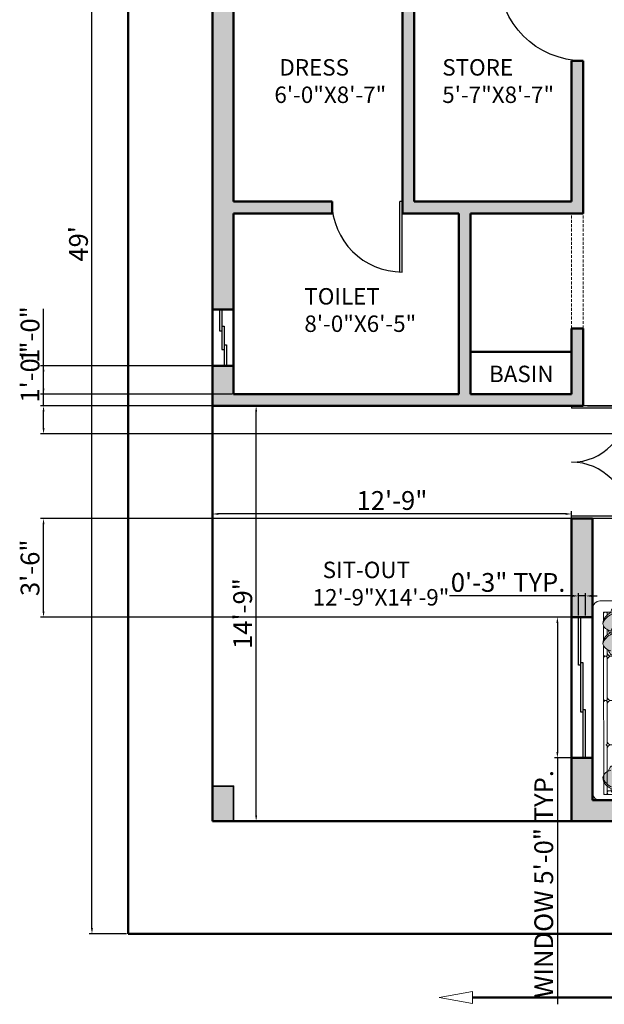
# Model space of a CAD drawing. Units: inches. Extents: x 1913 to 5309, y 1003 to 1733.
# Tile 9 of 23: x 2601 to 2850, y 1069 to 1488. Entities that reach past the tile are written whole.
import ezdxf

# ---------------------------------------------------------------- set-up
doc = ezdxf.new("R2010")
doc.units = ezdxf.units.IN
doc.linetypes.add('HIDDEN2', pattern=[0.1875, 0.125, -0.0625])
for name, color, linetype, lineweight in [('A-ANNO-DIMS', 2, 'Continuous', 18), ('A-ANNO-SYMB', 1, 'Continuous', 18), ('A-AREA-IDEN', 3, 'Continuous', 18), ('A-COLS', 5, 'Continuous', 35), ('A-COLS-PATT', 5, 'Continuous', 13), ('A-DOOR', 4, 'Continuous', 25), ('A-FLOR-PATT', 252, 'Continuous', 13), ('A-FURN', 8, 'Continuous', 18), ('A-GLAZ', 5, 'Continuous', 25), ('A-WALL', 7, 'Continuous', 50), ('A-WALL-OVHD', 8, 'HIDDEN2', 18)]:
    doc.layers.add(name, color=color, linetype=linetype, lineweight=lineweight)
doc.styles.get("Standard").update_dxf_attribs({"font": 'arial.ttf'})
doc.dimstyles.new('ISO-25', dxfattribs={"dimtxt": 8, "dimasz": 2.5, "dimexe": 1.25, "dimexo": 0.625, "dimtad": 1, "dimdec": 1, "dimlunit": 3, "dimtxsty": 'Standard', "dimcen": 2.5, "dimclrd": 256, "dimclrt": 1, "dimadec": 0, "dimazin": 0, "dimtfac": 1, "dimtdec": 1, "dimtmove": 0, "dimatfit": 3, "dimfxl": 1, "dimarcsym": 0})

# ---------------------------------------------------------------- blocks, each defined once
blk = doc.blocks.new('SOFA 1')
at = {"transparency": 33554687}
h = blk.add_hatch(color=256, dxfattribs=at)
h.dxf.hatch_style = 1
h.paths.add_polyline_path([(3723.52, 1308.63, 0.147724), (3717.76, 1305.24, 0.310469), (3722.42, 1300.4), (3722.42, 1300.25, 0.156703), (3723.62, 1297.8, 0.425821), (3734.69, 1309.08, 0.121928), (3732.05, 1310.63, 0.233216), (3728.6, 1313.59, 0.213835)])
h = blk.add_hatch(color=256, dxfattribs=at)
h.dxf.hatch_style = 1
h.paths.add_polyline_path([(3769.65, 1307.6, 0.084911), (3767.15, 1309.12, 0.046133), (3766.46, 1311.13), (3759.18, 1311.13, 0.039409), (3758.92, 1310.24, 0.165523), (3756.31, 1309.02, 0.42585), (3767.59, 1297.95, 0.121928), (3769.15, 1300.58, 0.027403), (3769.65, 1300.83)])
h.paths.add_polyline_path([(3765.34, 1313.08), (3760.4, 1313.08, 0.097704), (3759.18, 1311.13), (3766.46, 1311.13, 0.04873)])
h.paths.add_polyline_path([(3763.76, 1314.88, 0.16488), (3760.4, 1313.08), (3765.34, 1313.08, 0.051917)])
h.paths.add_polyline_path([(3771.6, 1305.17, 0.090388), (3769.65, 1307.6), (3769.65, 1300.83, 0.136035), (3771.6, 1302.77)])
h = blk.add_hatch(color=256, dxfattribs=at)
h.dxf.hatch_style = 1
h.paths.add_polyline_path([(3769.16, 1235.96, 0.122267), (3767.6, 1238.61, 0.425972), (3756.32, 1227.54, 0.165563), (3758.93, 1226.32, 0.309481), (3763.76, 1221.69, 0.002677), (3763.83, 1221.72, 0.146094), (3767.16, 1227.43, 0.212433), (3772.1, 1232.48, 0.235342)])
h = blk.add_hatch(color=256, dxfattribs=at)
h.dxf.hatch_style = 1
h.paths.add_polyline_path([(3769.16, 1225.36, 0.122267), (3767.6, 1228.01, 0.425972), (3756.32, 1216.94, 0.165563), (3758.93, 1215.72, 0.309481), (3763.76, 1211.09, 0.002677), (3763.83, 1211.12, 0.146094), (3767.16, 1216.83, 0.212433), (3772.1, 1221.88, 0.235342)])
for p, q in [((3720.45, 1316.13), (3773.58, 1316.13)), ((3777.51, 1312.19), (3777.51, 1213.72))]:
    blk.add_line(p, q, dxfattribs=at)
for points in [[(3717.76, 1305.24, -0.147724), (3723.52, 1308.63, -0.213355), (3728.59, 1313.59, 0.213355), (3723.52, 1308.63, 0.147724), (3717.76, 1305.24, -0.249545), (3722.86, 1309.34, 0.249545), (3717.75, 1305.25, 0.356779), (3723.4, 1300.28, -0.356779), (3717.76, 1305.24)], [(3728.58, 1313.6, -0.306333), (3732.42, 1309.31, 0.306333), (3728.58, 1313.6, 0.306674), (3722.72, 1308.89, -0.306674), (3728.58, 1313.6)], [(3763.76, 1314.88, -0.147724), (3767.15, 1309.12, -0.213355), (3772.1, 1304.05, 0.213355), (3767.15, 1309.12, 0.147724), (3763.76, 1314.88, -0.249545), (3767.86, 1309.77, 0.249545), (3763.77, 1314.89, 0.356779), (3758.8, 1309.23, -0.356779), (3763.76, 1314.88)], [(3734.69, 1309.08, -0.425972), (3723.62, 1297.8, -0.165552), (3722.4, 1300.4, 0.165552), (3723.62, 1297.79, 0.425972), (3734.69, 1309.07, 0.121514), (3732.07, 1310.63, -0.121514), (3734.69, 1309.08)], [(3767.6, 1297.95, -0.425972), (3756.31, 1309.01, -0.165552), (3758.92, 1310.24, 0.165552), (3756.31, 1309.02, 0.425972), (3767.59, 1297.95, 0.121514), (3769.14, 1300.57, -0.121514), (3767.6, 1297.95)], [(3772.11, 1304.06, -0.306333), (3767.83, 1300.22, 0.306333), (3772.11, 1304.06, 0.306674), (3767.4, 1309.91, -0.306674), (3772.11, 1304.06)], [(3770.44, 1286.63, -0.414214), (3769.66, 1287.4, 0.414214), (3770.44, 1286.63, 0.414214), (3769.66, 1285.83, -0.414214), (3770.44, 1286.63)], [(3748.01, 1262.99, -0.414214), (3746.05, 1264.95, 0.414214), (3748.01, 1262.97, 0.414213), (3746.05, 1261.01, -0.414213), (3748.01, 1262.99)], [(3770.44, 1262.99, -0.414214), (3769.66, 1263.77, 0.414214), (3770.44, 1262.99, 0.414214), (3769.66, 1262.19, -0.414214), (3770.44, 1262.99)], [(3770.83, 1262.97, -0.414214), (3771.61, 1262.19, 0.414214), (3770.83, 1262.99, 0.414214), (3771.61, 1263.77, -0.414214), (3770.83, 1262.97)], [(3748.01, 1239.35, -0.414214), (3746.05, 1241.31, 0.414214), (3748.01, 1239.33, 0.414213), (3746.05, 1237.37, -0.414213), (3748.01, 1239.35)], [(3767.7, 1239.33, -0.414214), (3769.66, 1237.37, 0.414214), (3767.7, 1239.35, 0.414214), (3769.66, 1241.31, -0.414214), (3767.7, 1239.33)], [(3770.44, 1239.35, -0.414214), (3769.66, 1240.13, 0.414214), (3770.44, 1239.33, 0.414214), (3769.66, 1238.55, -0.414214), (3770.44, 1239.35)], [(3770.83, 1239.33, -0.414214), (3771.61, 1238.55, 0.414214), (3770.83, 1239.35, 0.414214), (3771.61, 1240.13, -0.414214), (3770.83, 1239.33)], [(3756.32, 1227.54, -0.425972), (3767.6, 1238.61, -0.121514), (3769.16, 1235.98, 0.121514), (3767.6, 1238.61, 0.425972), (3756.32, 1227.54, 0.165552), (3758.93, 1226.32, -0.165552), (3756.32, 1227.54)], [(3772.1, 1232.5, -0.306674), (3767.41, 1226.64, 0.306674), (3772.1, 1232.5, 0.306333), (3767.84, 1236.34, -0.306333), (3772.1, 1232.5)], [(3763.78, 1221.67, 0.249545), (3767.87, 1226.78, -0.249545), (3763.76, 1221.69, -0.356779), (3758.81, 1227.32, 0.356779), (3763.77, 1221.68, 0.147724), (3767.16, 1227.43, 0.213355), (3772.11, 1232.51, -0.213355), (3767.16, 1227.43, -0.147724), (3763.78, 1221.67)], [(3756.32, 1216.94, -0.200233), (3759.49, 1224.76, 0.200233), (3756.32, 1216.94, 0.165552), (3758.93, 1215.72, -0.165552), (3756.32, 1216.94)], [(3772.1, 1221.9, -0.306674), (3767.41, 1216.04, 0.306674), (3772.1, 1221.9, -0.213355), (3767.16, 1216.83, -0.147724), (3763.77, 1211.08, 0.147724), (3767.15, 1216.83, 0.213355), (3772.1, 1221.9)], [(3763.76, 1211.09, -0.356779), (3758.81, 1216.72, 0.356779), (3763.76, 1211.09, 0.249545), (3767.87, 1216.18, -0.249545), (3763.76, 1211.09)]]:
    blk.add_lwpolyline(points, format="xyb", dxfattribs=at)
for points in [[(3716.51, 1312.2), (3716.51, 1291.44)], [(3722.42, 1313.08), (3722.42, 1309.23), (3722.42, 1313.08), (3726.57, 1313.08)], [(3723.21, 1311.13), (3723.93, 1311.13)], [(3729.85, 1313.08), (3745.25, 1313.08)], [(3731.82, 1311.13), (3745.25, 1311.13)], [(3746.01, 1312.3), (3746.01, 1288.55)], [(3746.01, 1310.97), (3746.01, 1311.36)], [(3746.01, 1288.54), (3746.01, 1308.23)], [(3768.11, 1313.08), (3746.78, 1313.08)], [(3768.87, 1311.13), (3746.78, 1311.13)], [(3771.6, 1313.08), (3767.75, 1313.08), (3771.6, 1313.08), (3771.6, 1308.93)], [(3769.66, 1287.39), (3769.65, 1312.3)], [(3769.65, 1309.43), (3769.65, 1308.71)], [(3771.6, 1313.08), (3771.61, 1233.74)], [(3722.42, 1300.39), (3722.42, 1297.33)], [(3720.45, 1295.38), (3718.48, 1295.38)], [(3720.45, 1287.5), (3744.09, 1287.5)], [(3746.02, 1284.63), (3746.02, 1264.94)], [(3747.99, 1286.6), (3767.69, 1286.6)], [(3769.66, 1263.75), (3769.66, 1285.81)], [(3769.66, 1277.18), (3769.66, 1263.75)], [(3746.02, 1260.99), (3746.02, 1241.3)], [(3747.99, 1262.97), (3767.69, 1262.97)], [(3769.66, 1240.12), (3769.66, 1262.18)], [(3770.43, 1262.97), (3770.82, 1262.97)], [(3746.02, 1237.36), (3746.02, 1213.74)], [(3747.99, 1239.33), (3767.69, 1239.33)], [(3769.66, 1235.71), (3769.66, 1238.54)], [(3770.43, 1239.33), (3770.82, 1239.33)], [(3771.61, 1223.14), (3771.61, 1230.47)], [(3769.66, 1225.11), (3769.66, 1227.82)], [(3767.76, 1215.72), (3771.61, 1215.72), (3771.61, 1219.84), (3771.61, 1215.72)], [(3753.91, 1211.77), (3753.91, 1213.74)], [(3755.86, 1215.72), (3758.92, 1215.72)], [(3769.66, 1216.5), (3769.66, 1217.22)], [(3749.97, 1209.8), (3773.58, 1209.8)]]:
    blk.add_lwpolyline(points, close=True, dxfattribs=at)
for points in [[(3722.42, 1311.91, 0.414214), (3723.2, 1311.13, -0.414214)], [(3770.43, 1313.08, 0.414214), (3769.65, 1312.3, -0.414214)], [(3771.6, 1312.3, 0.414214), (3770.82, 1313.08, -0.414214)], [(3716.51, 1297.34, 0.414214), (3718.47, 1295.38, -0.414214)], [(3720.44, 1295.38, 0.414214), (3722.4, 1297.34, -0.414214)], [(3716.51, 1291.45, 0.414212), (3720.44, 1287.52, -0.414212)], [(3746.03, 1288.56, 0.414214), (3747.99, 1286.6, 0.414213), (3746.03, 1284.64, -0.414213), (3747.99, 1286.6, -0.414214)], [(3769.66, 1284.64, 0.414214), (3767.7, 1286.6, 0.414214), (3769.66, 1288.56, -0.414214), (3767.7, 1286.6, -0.414214)], [(3769.66, 1261.01, 0.414214), (3767.7, 1262.97, 0.414214), (3769.66, 1264.93, -0.414214), (3767.7, 1262.97, -0.414214)], [(3772.13, 1221.9, 0.306333), (3767.84, 1225.74, -0.306333)], [(3769.16, 1225.36, 0.071861), (3768.39, 1227.01, -0.071861)], [(3746.05, 1213.76, 0.414212), (3749.98, 1209.82, -0.414212)], [(3755.87, 1215.72, 0.414214), (3753.91, 1213.76, -0.414214)], [(3769.66, 1216.52, 0.414214), (3770.44, 1215.74, -0.414214)], [(3770.83, 1215.74, 0.414214), (3771.61, 1216.52, -0.414214)], [(3755.87, 1209.8, -0.414214), (3753.91, 1211.76, 0.414214)]]:
    blk.add_lwpolyline(points, format="xyb", close=True, dxfattribs=at)
for centre, radius, start, end in [((3720.44, 1312.2), 3.93, 90.0002, 179.9998), ((3720.44, 1312.19), 3.94, 89.9158, 179.9154), ((3773.58, 1312.2), 3.93, 0.0002, 89.9998), ((3773.57, 1312.19), 3.94, 359.9158, 89.9154), ((3744.09, 1309.21), 1.92, 358.766, 90.5111), ((3745.22, 1312.29), 0.789, 0.8425, 90.8425), ((3745.24, 1311.91), 0.777, 270, 0), ((3745.24, 1311.91), 0.777, 270, 0), ((3746.8, 1312.29), 0.789, 89.1575, 179.1575), ((3746.79, 1311.91), 0.777, 180, 270), ((3746.79, 1311.91), 0.777, 180, 270), ((3747.93, 1309.21), 1.92, 89.4889, 181.234), ((3768.87, 1312.3), 0.777, 360, 90), ((3768.87, 1311.91), 0.777, 270, 0), ((3744.08, 1289.48), 1.96, 270, 360), ((3744.08, 1289.48), 1.96, 270, 360), ((3773.58, 1213.73), 3.93, 270.0002, 359.9998), ((3773.59, 1213.73), 3.93, 269.9156, 359.9152)]:
    blk.add_arc(centre, radius, start, end, dxfattribs=at)
blk = doc.blocks.new('*D41')
at = {"layer": 'A-ANNO-DIMS', "color": 0, "lineweight": -2, "transparency": 16777216}
for p, q in [((2646.71, 1686.96), (2630.73, 1686.96)), ((2631.98, 1101.46), (2631.98, 1684.46)), ((2646.71, 1098.96), (2630.73, 1098.96))]:
    blk.add_line(p, q, dxfattribs=at)
at = {"layer": 'A-ANNO-DIMS', "color": 0, "transparency": 16777216}
for points in [[(2631.56, 1684.46), (2632.4, 1684.46), (2631.98, 1686.96)], [(2631.56, 1101.46), (2632.4, 1101.46), (2631.98, 1098.96)]]:
    blk.add_solid(points, dxfattribs=at)
at = {"layer": 'Defpoints', "color": 0, "transparency": 16777216}
for p in [(2631.98, 1686.96), (2647.34, 1686.96), (2647.34, 1098.96)]:
    blk.add_point(p, dxfattribs=at)
at = {"layer": 'A-ANNO-DIMS', "color": 0, "transparency": 16777216, "insert": (2627.27, 1392.96), "char_height": 8, "attachment_point": 5, "rotation": 90}
blk.add_mtext("49'", dxfattribs=at)
blk = doc.blocks.new('*D46')
at = {"layer": 'A-ANNO-DIMS', "color": 0, "lineweight": -2, "transparency": 16777216}
for p, q in [((2701.39, 1323.96), (2703.2, 1323.96)), ((2701.95, 1149.46), (2701.95, 1321.46)), ((2701.39, 1146.96), (2703.2, 1146.96))]:
    blk.add_line(p, q, dxfattribs=at)
at = {"layer": 'A-ANNO-DIMS', "color": 0, "transparency": 16777216}
for points in [[(2701.54, 1321.46), (2702.37, 1321.46), (2701.95, 1323.96)], [(2701.54, 1149.46), (2702.37, 1149.46), (2701.95, 1146.96)]]:
    blk.add_solid(points, dxfattribs=at)
at = {"layer": 'Defpoints', "color": 0, "transparency": 16777216}
for p in [(2700.77, 1323.96), (2701.95, 1323.96), (2700.77, 1146.96)]:
    blk.add_point(p, dxfattribs=at)
at = {"layer": 'A-ANNO-DIMS', "color": 0, "transparency": 16777216, "insert": (2697.24, 1235.46), "char_height": 8, "attachment_point": 5, "rotation": 90}
blk.add_mtext('14\'-9"', dxfattribs=at)
blk = doc.blocks.new('*D47')
at = {"layer": 'A-ANNO-DIMS', "color": 0, "lineweight": -2, "transparency": 16777216}
for p, q in [((2683.34, 1276.59), (2683.34, 1279.13)), ((2833.84, 1277.88), (2685.84, 1277.88)), ((2836.34, 1276.59), (2836.34, 1279.13))]:
    blk.add_line(p, q, dxfattribs=at)
at = {"layer": 'A-ANNO-DIMS', "color": 0, "transparency": 16777216}
for points in [[(2685.84, 1278.3), (2685.84, 1277.47), (2683.34, 1277.88)], [(2833.84, 1278.3), (2833.84, 1277.47), (2836.34, 1277.88)]]:
    blk.add_solid(points, dxfattribs=at)
at = {"layer": 'Defpoints', "color": 0, "transparency": 16777216}
for p in [(2683.34, 1277.88), (2683.34, 1275.96), (2836.34, 1275.96)]:
    blk.add_point(p, dxfattribs=at)
at = {"layer": 'A-ANNO-DIMS', "color": 0, "transparency": 16777216, "insert": (2759.84, 1282.59), "char_height": 8, "attachment_point": 5}
blk.add_mtext('12\'-9"', dxfattribs=at)
blk = doc.blocks.new('*D49')
at = {"layer": 'A-ANNO-DIMS', "color": 0, "lineweight": -2, "transparency": 16777216}
for p, q in [((2841.34, 1324.59), (2841.34, 1325.21)), ((2843.84, 1323.96), (3026.84, 1323.96)), ((3029.34, 1324.59), (3029.34, 1325.21))]:
    blk.add_line(p, q, dxfattribs=at)
at = {"layer": 'A-ANNO-DIMS', "color": 0, "transparency": 16777216}
for points in [[(2843.84, 1324.38), (2843.84, 1323.55), (2841.34, 1323.96)], [(3026.84, 1324.38), (3026.84, 1323.55), (3029.34, 1323.96)]]:
    blk.add_solid(points, dxfattribs=at)
at = {"layer": 'Defpoints', "color": 0, "transparency": 16777216}
for p in [(2841.34, 1323.96), (3029.34, 1323.96), (3029.34, 1323.96)]:
    blk.add_point(p, dxfattribs=at)
at = {"layer": 'A-ANNO-DIMS', "color": 0, "transparency": 16777216, "insert": (2935.34, 1328.67), "char_height": 8, "attachment_point": 5}
blk.add_mtext('15\'-8"', dxfattribs=at)
blk = doc.blocks.new("MD D 4'")
for p, q in [((0, 24), (0, 0)), ((1, 24), (1, 0)), ((47, 24), (47, 0)), ((48, 24), (48, 0)), ((0, 0), (1, 0)), ((48, 0), (47, 0))]:
    blk.add_line(p, q)
for centre, start, end in [((0, 0), 0, 90), ((48, 0), 90, 180)]:
    blk.add_arc(centre, 24, start, end)
blk = doc.blocks.new("D2 2'6")
for p, q in [((0, 30), (0, 0)), ((1, 30), (1, 0)), ((0, 0), (1, 0))]:
    blk.add_line(p, q)
blk.add_arc((0, 0), 30, 0, 90)
blk = doc.blocks.new("D1 3'")
for p, q in [((0, 36), (0, 0)), ((1, 36), (1, 0)), ((0, 0), (1, 0))]:
    blk.add_line(p, q)
blk.add_arc((0, 0), 36, 0, 90)
blk = doc.blocks.new('WIN-24')
for p, q in [((0, 15), (0, 24)), ((1, 7), (1, 24)), ((2, 17), (1, 17)), ((2, 0), (2, 17)), ((1, 15), (0, 15)), ((3, 9), (2, 9)), ((3, 0), (3, 9)), ((2, 7), (1, 7))]:
    blk.add_line(p, q)
blk = doc.blocks.new('WIN-60')
for p, q in [((0, 60), (0, 39.5)), ((1, 60), (1, 19.5)), ((0, 39.5), (1, 39.5)), ((1, 40.5), (2, 40.5)), ((2, 40.5), (2, 0)), ((1, 19.5), (2, 19.5)), ((2, 20.5), (3, 20.5)), ((3, 20.5), (3, 0))]:
    blk.add_line(p, q)
blk = doc.blocks.new('*D75')
at = {"layer": 'A-ANNO-DIMS', "color": 0, "lineweight": -2, "transparency": 16777216}
for p, q in [((2838.71, 1233.96), (2829.09, 1233.96)), ((2838.71, 1173.96), (2829.09, 1173.96))]:
    blk.add_line(p, q, dxfattribs=at)
at = {"layer": 'A-ANNO-DIMS', "lineweight": -2, "transparency": 16777216}
for p, q in [((2830.34, 1231.46), (2830.34, 1176.46)), ((2830.34, 1173.96), (2830.34, 1068.98))]:
    blk.add_line(p, q, dxfattribs=at)
at = {"layer": 'A-ANNO-DIMS', "transparency": 16777216}
for points in [[(2829.92, 1231.46), (2830.76, 1231.46), (2830.34, 1233.96)], [(2829.92, 1176.46), (2830.76, 1176.46), (2830.34, 1173.96)]]:
    blk.add_solid(points, dxfattribs=at)
at = {"layer": 'Defpoints', "color": 0, "transparency": 16777216}
for p in [(2839.34, 1233.96), (2830.34, 1173.96), (2839.34, 1173.96)]:
    blk.add_point(p, dxfattribs=at)
at = {"layer": 'A-ANNO-DIMS', "color": 1, "transparency": 16777216, "insert": (2825.57, 1120.22), "char_height": 8, "attachment_point": 5, "rotation": 90}
blk.add_mtext('WINDOW 5\'-0" TYP.', dxfattribs=at)
blk = doc.blocks.new('*D76')
at = {"layer": 'A-ANNO-DIMS', "lineweight": -2, "transparency": 16777216}
for p, q in [((2836.84, 1242.96), (2784.32, 1242.96)), ((2842.34, 1242.96), (2839.34, 1242.96)), ((2844.84, 1242.96), (2847.34, 1242.96))]:
    blk.add_line(p, q, dxfattribs=at)
at = {"layer": 'A-ANNO-DIMS', "color": 0, "lineweight": -2, "transparency": 16777216}
for p, q in [((2839.34, 1234.59), (2839.34, 1244.21)), ((2842.34, 1234.59), (2842.34, 1244.21))]:
    blk.add_line(p, q, dxfattribs=at)
at = {"layer": 'A-ANNO-DIMS', "transparency": 16777216}
for points in [[(2836.84, 1243.38), (2836.84, 1242.55), (2839.34, 1242.96)], [(2844.84, 1243.38), (2844.84, 1242.55), (2842.34, 1242.96)]]:
    blk.add_solid(points, dxfattribs=at)
at = {"layer": 'Defpoints', "color": 0, "transparency": 16777216}
for p in [(2839.34, 1242.96), (2839.34, 1233.96), (2842.34, 1233.96)]:
    blk.add_point(p, dxfattribs=at)
at = {"layer": 'A-ANNO-DIMS', "color": 1, "transparency": 16777216, "insert": (2809.33, 1247.68), "char_height": 8, "attachment_point": 5}
blk.add_mtext('0\'-3" TYP.', dxfattribs=at)
blk = doc.blocks.new('*D119')
at = {"layer": 'A-ANNO-DIMS', "lineweight": -2, "transparency": 16777216}
for p, q in [((2611.34, 1340.96), (2611.34, 1365.23)), ((2611.34, 1331.46), (2611.34, 1338.46))]:
    blk.add_line(p, q, dxfattribs=at)
at = {"layer": 'A-ANNO-DIMS', "color": 0, "lineweight": -2, "transparency": 16777216}
for p, q in [((2691.71, 1340.96), (2610.09, 1340.96)), ((2691.71, 1328.96), (2610.09, 1328.96))]:
    blk.add_line(p, q, dxfattribs=at)
at = {"layer": 'A-ANNO-DIMS', "transparency": 16777216}
for points in [[(2610.92, 1338.46), (2611.76, 1338.46), (2611.34, 1340.96)], [(2610.92, 1331.46), (2611.76, 1331.46), (2611.34, 1328.96)]]:
    blk.add_solid(points, dxfattribs=at)
at = {"layer": 'Defpoints', "color": 0, "transparency": 16777216}
for p in [(2611.34, 1340.96), (2692.34, 1340.96), (2692.34, 1328.96)]:
    blk.add_point(p, dxfattribs=at)
at = {"layer": 'A-ANNO-DIMS', "color": 1, "transparency": 16777216, "insert": (2606.63, 1354.35), "char_height": 8, "attachment_point": 5, "rotation": 90}
blk.add_mtext('1\'-0"', dxfattribs=at)
blk = doc.blocks.new('*D125')
at = {"layer": 'A-ANNO-DIMS', "color": 0, "lineweight": -2, "transparency": 16777216}
for p, q in [((2844.71, 1275.96), (2610.09, 1275.96)), ((2844.71, 1233.96), (2610.09, 1233.96))]:
    blk.add_line(p, q, dxfattribs=at)
at = {"layer": 'A-ANNO-DIMS', "lineweight": -2, "transparency": 16777216}
blk.add_line((2611.34, 1236.46), (2611.34, 1273.46), dxfattribs=at)
at = {"layer": 'A-ANNO-DIMS', "transparency": 16777216}
for points in [[(2610.92, 1273.46), (2611.76, 1273.46), (2611.34, 1275.96)], [(2610.92, 1236.46), (2611.76, 1236.46), (2611.34, 1233.96)]]:
    blk.add_solid(points, dxfattribs=at)
at = {"layer": 'Defpoints', "color": 0, "transparency": 16777216}
for p in [(2611.34, 1275.96), (2845.34, 1275.96), (2845.34, 1233.96)]:
    blk.add_point(p, dxfattribs=at)
at = {"layer": 'A-ANNO-DIMS', "color": 1, "transparency": 16777216, "insert": (2606.63, 1254.96), "char_height": 8, "attachment_point": 5, "rotation": 90}
blk.add_mtext('3\'-6"', dxfattribs=at)
blk = doc.blocks.new('*D127')
at = {"layer": 'A-ANNO-DIMS', "lineweight": -2, "transparency": 16777216}
for p, q in [((2611.34, 1323.96), (2611.34, 1348.23)), ((2611.34, 1314.46), (2611.34, 1321.46))]:
    blk.add_line(p, q, dxfattribs=at)
at = {"layer": 'A-ANNO-DIMS', "color": 0, "lineweight": -2, "transparency": 16777216}
for p, q in [((3033.71, 1323.96), (2610.09, 1323.96)), ((3028.71, 1311.96), (2610.09, 1311.96))]:
    blk.add_line(p, q, dxfattribs=at)
at = {"layer": 'A-ANNO-DIMS', "transparency": 16777216}
for points in [[(2610.92, 1321.46), (2611.76, 1321.46), (2611.34, 1323.96)], [(2610.92, 1314.46), (2611.76, 1314.46), (2611.34, 1311.96)]]:
    blk.add_solid(points, dxfattribs=at)
at = {"layer": 'Defpoints', "color": 0, "transparency": 16777216}
for p in [(2611.34, 1323.96), (3034.34, 1323.96), (3029.34, 1311.96)]:
    blk.add_point(p, dxfattribs=at)
at = {"layer": 'A-ANNO-DIMS', "color": 1, "transparency": 16777216, "insert": (2606.63, 1337.35), "char_height": 8, "attachment_point": 5, "rotation": 90}
blk.add_mtext('1\'-0"', dxfattribs=at)

msp = doc.modelspace()

# ---------------------------------------------------------------- hatches: boundary and pattern name
at = {"layer": 'A-COLS-PATT'}
h = msp.add_hatch(color=256, dxfattribs=at)
h.dxf.hatch_style = 1
h.paths.add_polyline_path([(2692.34, 1161.96), (2683.34, 1161.96), (2683.34, 1146.96), (2692.34, 1146.96)])
at = {"layer": 'A-FLOR-PATT'}
h = msp.add_hatch(color=256, dxfattribs=at)
h.dxf.hatch_style = 1
h.paths.add_polyline_path([(2841.34, 1686.96), (2683.34, 1686.96), (2683.34, 1625.96), (2692.34, 1625.96), (2692.34, 1677.96), (2836.34, 1677.96), (2836.34, 1554.96), (2841.34, 1554.96), (2841.34, 1599.96), (2859.31, 1599.96), (2859.31, 1608.96), (2841.34, 1608.96)])
h.paths.add_polyline_path([(3034.34, 1625.46), (3029.34, 1625.46), (3029.34, 1608.96), (2955.31, 1608.96), (2955.31, 1599.96), (3029.34, 1599.96), (3029.34, 1528.96), (3034.34, 1528.96)])
h.paths.add_polyline_path([(3199.34, 1686.96), (3029.34, 1686.96), (3029.34, 1661.46), (3034.34, 1661.46), (3034.34, 1677.96), (3190.34, 1677.96), (3190.34, 1492.96), (3029.34, 1492.96), (3029.34, 1487.96), (3158.34, 1487.96), (3158.34, 1464.96), (3163.34, 1464.96), (3163.34, 1487.96), (3199.34, 1487.96)])
h.paths.add_polyline_path([(3099.34, 1400.96), (3163.34, 1400.96), (3163.34, 1428.96), (3158.34, 1428.96), (3158.34, 1405.96), (3029.34, 1405.96), (3029.34, 1311.96), (3034.34, 1311.96), (3034.34, 1323.96), (3058.34, 1323.96), (3058.34, 1328.96), (3034.34, 1328.96), (3034.34, 1400.96), (3094.34, 1400.96), (3094.34, 1358.96), (3099.34, 1358.96)])
h.paths.add_polyline_path([(3199.34, 1405.96), (3187.34, 1405.96), (3187.34, 1400.96), (3190.34, 1400.96), (3190.34, 1328.96), (3094.34, 1328.96), (3094.34, 1323.96), (3190.34, 1323.96), (3190.34, 1299.96), (3190.34, 1179.96), (3176.2, 1179.96), (3139.34, 1179.96), (3139.34, 1170.96), (3190.34, 1170.96), (3190.34, 1146.96), (3199.34, 1146.96)])
h.paths.add_polyline_path([(3085.34, 1179.96), (3064.34, 1179.96), (3064.34, 1170.96), (3085.34, 1170.96)])
h.paths.add_polyline_path([(3029.34, 1158.98), (3029.34, 1199.59, 0.414216), (3026.32, 1202.59), (3010.47, 1202.59, 0.414214), (3007.47, 1199.59), (3007.47, 1181.52, 0.46174), (3009.2, 1180.04), (3026.11, 1180.04, 0.414263), (3025.52, 1179.45), (3025.52, 1162.57, 0.41435), (3026.11, 1161.97), (3007.38, 1161.97, 0.41842), (3006.78, 1161.36, 0.785879), (3005.87, 1162.09, 0.298637), (3006.77, 1163.46), (3006.77, 1178.53, 0.414214), (3005.27, 1180.02), (2990.22, 1180.02, 0.416116), (2988.72, 1178.51, 0.414208), (2987.21, 1180.02), (2987.2, 1180.02, -0.413869), (2988.7, 1178.52, -0.412492), (2990.21, 1180.02), (2990.21, 1180.03), (3005.27, 1180.02, -0.414213), (3006.77, 1178.53, -0.414214), (3008.27, 1180.02), (3008.14, 1180.27, -0.252555), (3007.47, 1181.52), (3007.45, 1181.51), (3007.47, 1199.59, -0.414214), (3010.47, 1202.59), (3026.33, 1202.59, -0.414214), (3029.34, 1199.59), (3029.34, 1275.96), (3034.34, 1275.96), (3034.34, 1146.96), (3011.34, 1146.96), (3011.34, 1155.96), (2951.06, 1155.96, -0.414214), (2948.06, 1158.97), (2948.06, 1158.97, 0.421637), (2951.14, 1155.96), (3026.4, 1155.96, 0.407251)])
h.paths.add_polyline_path([(2845.34, 1275.96), (2836.34, 1275.96), (2836.34, 1233.96), (2845.34, 1233.96), (2845.34, 1237.71)])
h.paths.add_polyline_path([(2845.34, 1173.96), (2836.34, 1173.96), (2836.34, 1146.96), (2863.34, 1146.96), (2863.34, 1155.93), (2848.48, 1155.93, -0.414214), (2845.34, 1159.07)])
h.paths.add_polyline_path([(2841.34, 1356.96), (2836.34, 1356.96), (2836.34, 1328.96), (2793.34, 1328.96), (2793.34, 1405.96), (2841.34, 1405.96), (2841.34, 1470.96), (2836.34, 1470.96), (2836.34, 1410.96), (2769.34, 1410.96), (2769.34, 1513.96), (2836.34, 1513.96), (2836.34, 1506.96), (2841.34, 1506.96), (2841.34, 1518.96), (2764.34, 1518.96), (2764.34, 1405.96), (2788.34, 1405.96), (2788.34, 1328.96), (2692.34, 1328.96), (2692.34, 1340.96), (2683.34, 1340.96), (2683.34, 1323.96), (2841.34, 1323.96)])
h.paths.add_polyline_path([(2692.34, 1513.96), (2734.34, 1513.96), (2734.34, 1518.96), (2692.34, 1518.96), (2692.34, 1571.96), (2683.34, 1571.96), (2683.34, 1420.96), (2683.34, 1364.96), (2692.34, 1364.96), (2692.34, 1405.96), (2734.34, 1405.96), (2734.34, 1410.96), (2692.34, 1410.96)])

# ---------------------------------------------------------------- linework, layer by layer
at = {"layer": 'A-ANNO-SYMB'}
msp.add_lwpolyline([(2780, 1071.84), (2794.16, 1074.39), (2794.16, 1069.29)], close=True, dxfattribs=at)
at = {"layer": 'A-COLS'}
msp.add_lwpolyline([(2683.34, 1146.96), (2692.34, 1146.96), (2692.34, 1161.96), (2683.34, 1161.96)], close=True, dxfattribs=at)
at = {"layer": 'A-WALL'}
for p, q in [((2647.34, 1098.96), (2647.34, 1686.96)), ((2683.34, 1686.96), (2683.34, 1420.96)), ((2764.34, 1518.96), (2764.34, 1405.96)), ((2692.34, 1513.96), (2692.34, 1410.96)), ((2769.34, 1513.96), (2769.34, 1410.96)), ((2836.34, 1470.96), (2836.34, 1410.96)), ((2836.34, 1470.96), (2841.34, 1470.96)), ((2841.34, 1470.96), (2841.34, 1405.96)), ((2683.34, 1420.96), (2683.34, 1146.96)), ((2734.34, 1410.96), (2692.34, 1410.96)), ((2734.34, 1410.96), (2734.34, 1405.96)), ((2836.34, 1410.96), (2769.34, 1410.96)), ((2692.34, 1405.96), (2692.34, 1328.96)), ((2734.34, 1405.96), (2692.34, 1405.96)), ((2788.34, 1405.96), (2764.34, 1405.96)), ((2788.34, 1405.96), (2788.34, 1328.96)), ((2841.34, 1405.96), (2793.34, 1405.96)), ((2793.34, 1405.96), (2793.34, 1328.96)), ((2683.34, 1364.96), (2692.34, 1364.96)), ((2836.34, 1356.96), (2841.34, 1356.96)), ((2836.34, 1356.96), (2836.34, 1328.96)), ((2841.34, 1356.96), (2841.34, 1323.96)), ((2836.34, 1346.96), (2793.34, 1346.96)), ((2683.34, 1340.96), (2692.34, 1340.96)), ((2788.34, 1328.96), (2692.34, 1328.96)), ((2836.34, 1328.96), (2793.34, 1328.96)), ((2841.34, 1323.96), (2683.34, 1323.96)), ((2836.34, 1275.96), (2836.34, 1146.96)), ((2845.34, 1275.96), (2836.34, 1275.96)), ((2845.34, 1275.96), (2845.34, 1155.96)), ((2836.34, 1233.96), (2845.34, 1233.96)), ((2836.34, 1173.96), (2845.34, 1173.96)), ((2845.34, 1155.96), (3029.34, 1155.96)), ((2836.34, 1146.96), (2683.34, 1146.96)), ((2836.34, 1146.96), (3199.34, 1146.96)), ((3199.34, 1098.96), (2647.34, 1098.96)), ((2794.16, 1071.84), (2893.98, 1071.84))]:
    msp.add_line(p, q, dxfattribs=at)
at = {"layer": 'A-WALL-OVHD', "ltscale": 10}
for p, q in [((2836.34, 1356.96), (2836.34, 1405.96)), ((2841.34, 1356.96), (2841.34, 1405.96))]:
    msp.add_line(p, q, dxfattribs=at)

# ---------------------------------------------------------------- block references
at = {"layer": 'A-DOOR', "xscale": -1, "rotation": 90}
msp.add_blockref("D1 3'", (2841.34, 1506.96), dxfattribs=at)
at = {"layer": 'A-DOOR'}
for name, p, rotation in [("D2 2'6", (2764.21, 1410.96), 180), ("MD D 4'", (2836.34, 1323.96), 270)]:
    msp.add_blockref(name, p, dxfattribs=dict(at, rotation=rotation))
at = {"layer": 'A-FURN', "xscale": 0.7985303345031592, "yscale": 0.7985303345031592, "zscale": 0.7985303345031592, "rotation": 180}
msp.add_blockref('SOFA 1', (5861.8, 2206.9), dxfattribs=at)
at = {"layer": 'A-GLAZ', "rotation": 180}
for name, p in [('WIN-24', (2689.34, 1364.96)), ('WIN-60', (2842.34, 1233.96))]:
    msp.add_blockref(name, p, dxfattribs=at)

# ---------------------------------------------------------------- texts
at = {"layer": 'A-AREA-IDEN', "char_height": 7, "attachment_point": 1}
for s, insert in [(' DRESS\\P6\'-0"X8\'-7"', (2709.73, 1471.66)), ('STORE\\P5\'-7"X8\'-7"', (2781.27, 1471.66)), ('TOILET\\P8\'-0"X6\'-5"', (2722.51, 1374.11)), ('BASIN', (2801.21, 1341.05)), ('  SIT-OUT\\P12\'-9"X14\'-9"', (2726.03, 1257.55))]:
    msp.add_mtext_dynamic_manual_height_columns(s, width=86.9528, gutter_width=12.5, heights=[0], dxfattribs=dict(at, insert=insert))

# ---------------------------------------------------------------- dimensions: what is measured, and where the dimension line sits
at = {"layer": 'A-ANNO-DIMS'}
for base, p1, p2, override, picture, middle in [((2631.98, 1686.96), (2647.34, 1098.96), (2647.34, 1686.96), {"dimclrd": 0, "dimclre": 0, "dimclrt": 0}, '*D41', (2627.27, 1392.96)), ((2611.34, 1340.96), (2692.34, 1328.96), (2692.34, 1340.96), {"dimdec": 1, "dimlfac": 1, "dimrnd": 0, "dimzin": 1, "dimdsep": 46, "dimlunit": 4, "dimfrac": 2}, '*D119', (2606.63, 1354.35)), ((2611.34, 1323.96), (3029.34, 1311.96), (3034.34, 1323.96), {"dimdec": 1, "dimlfac": 1, "dimrnd": 0, "dimzin": 1, "dimdsep": 46, "dimlunit": 4, "dimfrac": 2}, '*D127', (2606.63, 1337.35)), ((2701.95, 1323.96), (2700.77, 1146.96), (2700.77, 1323.96), {"dimclrd": 0, "dimclre": 0, "dimclrt": 0}, '*D46', (2697.24, 1235.46)), ((2611.34, 1275.96), (2845.34, 1233.96), (2845.34, 1275.96), {"dimdec": 1, "dimlfac": 1, "dimrnd": 0, "dimzin": 1, "dimdsep": 46, "dimlunit": 4, "dimfrac": 2}, '*D125', (2606.63, 1254.96))]:
    dim = msp.add_linear_dim(base=base, p1=p1, p2=p2, angle=90, dimstyle='ISO-25', override=override, dxfattribs=at)
    dim.commit()
    dim.dimension.update_dxf_attribs({"geometry": picture, "text_midpoint": middle})
for base, p1, p2, picture, middle in [((3029.34, 1323.96), (2841.34, 1323.96), (3029.34, 1323.96), '*D49', (2935.34, 1328.67)), ((2683.34, 1277.88), (2836.34, 1275.96), (2683.34, 1275.96), '*D47', (2759.84, 1282.59))]:
    dim = msp.add_linear_dim(base=base, p1=p1, p2=p2, dimstyle='ISO-25', override={"dimclrd": 0, "dimclre": 0, "dimclrt": 0}, dxfattribs=at)
    dim.commit()
    dim.dimension.update_dxf_attribs({"geometry": picture, "text_midpoint": middle})
for base, p1, p2, angle, text, picture, middle in [((2839.34, 1242.96), (2842.34, 1233.96), (2839.34, 1233.96), 180, '<> TYP.', '*D76', (2809.33, 1247.68)), ((2830.34, 1173.96), (2839.34, 1233.96), (2839.34, 1173.96), 270, 'WINDOW <> TYP.', '*D75', (2825.57, 1120.22))]:
    dim = msp.add_linear_dim(base=base, p1=p1, p2=p2, angle=angle, text=text, dimstyle='ISO-25', override={"dimdec": 1, "dimrnd": 0, "dimzin": 1, "dimlunit": 4, "dimfrac": 2}, dxfattribs=at)
    dim.commit()
    dim.dimension.update_dxf_attribs({"geometry": picture, "text_midpoint": middle})

doc.saveas('drawing.dxf')
